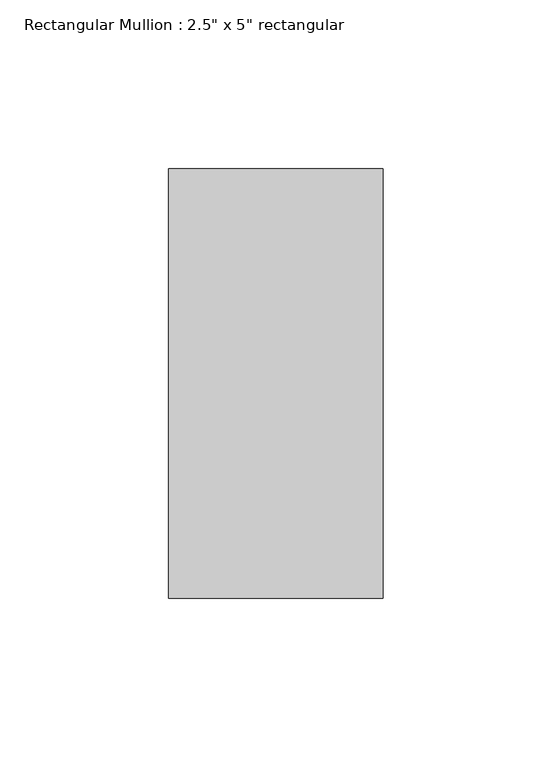
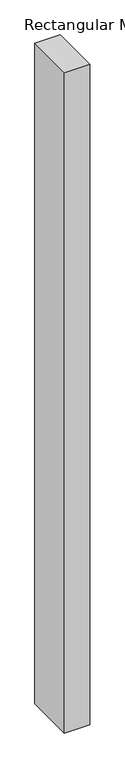
"""IFC4 building model written with IfcOpenShell, lengths in millimetres: member geometry."""

from ifc_helpers import new_model, si_unit, frame, origin, place, context, project, spatial, polyline, outline, extrude, source, transform, mapped, element, save


def member_dac5616b(model_context):
    return source(origin(), model_context, "Body", "SweptSolid", [
        extrude(outline(polyline([(31.75, 63.5), (31.75, -63.5), (-31.75, -63.5), (-31.75, 63.5), (31.75, 63.5)])), frame((0.0, 0.0, -1736.0162259), z_axis=(0.0, 0.0, 1.0), x_axis=(1.0, 0.0, 0.0)), (0.0, 0.0, 1.0), 1736.0162259),
    ])


if __name__ == "__main__":
    model = new_model("IFC4")
    model_context = context("Model", 3, world=origin())
    ifc_project = project(units=[si_unit("LENGTHUNIT", "METRE", prefix="MILLI")], contexts=[model_context])
    site = spatial("IfcSite", under=ifc_project)
    building = spatial("IfcBuilding", under=site)
    placement = place(None, origin())
    member_shape = member_dac5616b(model_context)
    element("IfcMember", 1, ObjectType="Rectangular Mullion : 2.5\" x 5\" rectangular", at=placement, inside=building, context=model_context, shape_type="MappedRepresentation", body=[
        mapped(member_shape, transform((0.0, 0.0, 0.0), x_axis=(1.0, 0.0, 0.0), y_axis=(0.0, 1.0, 0.0), z_axis=(0.0, 0.0, 1.0))),
    ])
    save(model, "model.ifc")

# Revit data of these elements
# Type "Rectangular Mullion : 2.5\" x 5\" rectangular"
#   built-in parameter 1007304 = 0.416667 (stored number, unit not read)
#   built-in parameter 1007301 = 0.104167 (stored number, unit not read)
#   built-in parameter 1007300 = 0.104167 (stored number, unit not read)
# Element 1 (IfcMember, "Rectangular Mullion : 2.5\" x 5\" rectangular")
#   Materials on its faces: "Aluminum"
# Materials
#   "Aluminum": class "Metal", colour RGB 247 247 247, transparency 0, Description = "Aluminum 6061", Cost = 0
